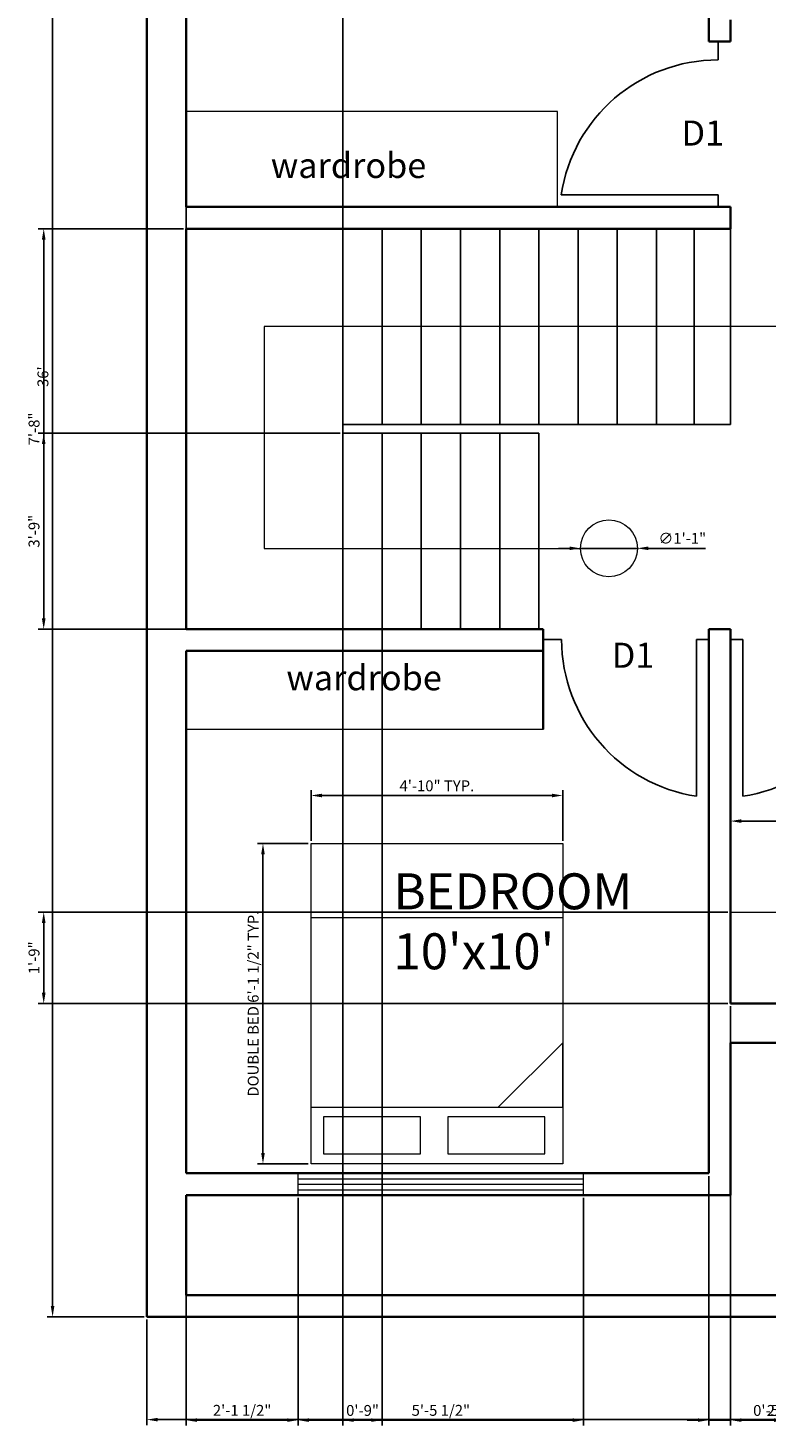
# Model space of a CAD drawing. Units: inches. Extents: x 346 to 762, y 179 to 666.
# Tile 1 of 3: x 348 to 518, y 179 to 500. Entities that reach past the tile are written whole.
import ezdxf

# ---------------------------------------------------------------- set-up
doc = ezdxf.new("R2010")
doc.units = ezdxf.units.IN
for name, color, linetype, lineweight in [('A-ANNO-DIMS', 2, 'Continuous', 18), ('A-ANNO-SYMB', 3, 'Continuous', 18), ('A-ANNO-TEXT', 7, 'Continuous', 18), ('A-AREA-IDEN', 7, 'Continuous', 25), ('A-DOOR', 3, 'Continuous', 25), ('A-FLOR-CASE', 9, 'Continuous', 18), ('A-FLOR-STRS', 7, 'Continuous', 25), ('A-FURN', 8, 'Continuous', 18), ('A-GLAZ', 4, 'Continuous', 18), ('A-WALL', 7, 'Continuous', 35)]:
    doc.layers.add(name, color=color, linetype=linetype, lineweight=lineweight)
doc.styles.get("Standard").update_dxf_attribs({"font": 'arial.ttf'})
doc.dimstyles.new('ISO-25', dxfattribs={"dimtxt": 2.5, "dimasz": 2.5, "dimexe": 1.25, "dimexo": 0.625, "dimtad": 1, "dimdec": 0, "dimlunit": 3, "dimtxsty": 'Standard', "dimcen": 2.5, "dimadec": 0, "dimazin": 0, "dimtfac": 1, "dimtdec": 0, "dimtmove": 0, "dimatfit": 3, "dimfxl": 1, "dimarcsym": 0})

# ---------------------------------------------------------------- blocks, each defined once
blk = doc.blocks.new('*D2')
at = {"layer": 'A-ANNO-DIMS', "color": 0, "lineweight": -2, "transparency": 16777216}
for p, q in [((375.04, 636.22), (352.75, 636.22)), ((354, 633.72), (354, 206.72)), ((375.04, 204.22), (352.75, 204.22))]:
    blk.add_line(p, q, dxfattribs=at)
at = {"layer": 'A-ANNO-DIMS', "color": 0, "transparency": 16777216}
for points in [[(353.58, 633.72), (354.41, 633.72), (354, 636.22)], [(353.58, 206.72), (354.41, 206.72), (354, 204.22)]]:
    blk.add_solid(points, dxfattribs=at)
at = {"layer": 'Defpoints', "color": 0, "transparency": 16777216}
for p in [(375.66, 636.22), (354, 204.22), (375.66, 204.22)]:
    blk.add_point(p, dxfattribs=at)
at = {"layer": 'A-ANNO-DIMS', "color": 0, "transparency": 16777216, "insert": (352.1, 420.22), "char_height": 2.5, "attachment_point": 5, "rotation": 90}
blk.add_mtext("36'", dxfattribs=at)
blk = doc.blocks.new('*D4')
at = {"layer": 'A-ANNO-DIMS', "color": 0, "lineweight": -2, "transparency": 16777216}
for p, q in [((375.66, 203.6), (375.66, 179.38)), ((735.66, 203.6), (735.66, 179.38)), ((378.16, 180.63), (733.16, 180.63))]:
    blk.add_line(p, q, dxfattribs=at)
at = {"layer": 'A-ANNO-DIMS', "color": 0, "transparency": 16777216}
for points in [[(378.16, 181.05), (378.16, 180.21), (375.66, 180.63)], [(733.16, 181.05), (733.16, 180.21), (735.66, 180.63)]]:
    blk.add_solid(points, dxfattribs=at)
at = {"layer": 'Defpoints', "color": 0, "transparency": 16777216}
for p in [(375.66, 204.22), (735.66, 204.22), (735.66, 180.63)]:
    blk.add_point(p, dxfattribs=at)
at = {"layer": 'A-ANNO-DIMS', "color": 0, "transparency": 16777216, "insert": (555.66, 182.53), "char_height": 2.5, "attachment_point": 5}
blk.add_mtext("30'", dxfattribs=at)
blk = doc.blocks.new('BED-DOUBLE')
for p, q in [((0, 0), (0, 73.56)), ((0, 73.56), (57.79, 73.56)), ((57.79, 73.56), (57.79, 0)), ((0, 56.59), (57.79, 56.59)), ((57.79, 27.81), (42.96, 13.04)), ((57.79, 13.04), (57.79, 27.81)), ((0, 0), (0, 13.04)), ((0, 13.04), (57.79, 13.04)), ((57.79, 0), (0, 0))]:
    blk.add_line(p, q)
for points in [[(2.87, 2.28), (25.15, 2.28), (25.15, 10.76), (2.87, 10.76)], [(31.41, 2.28), (53.7, 2.28), (53.7, 10.76), (31.41, 10.76)]]:
    blk.add_lwpolyline(points, close=True)
blk = doc.blocks.new('DOOR-SINGLE-36IN')
for p, q in [((2.79, 36), (0, 36)), ((2.79, 36), (2.79, 0)), ((38, 36), (33.78, 36))]:
    blk.add_line(p, q)
blk.add_arc((-2.63, 36), 36.41, 278.5676, 0)
blk = doc.blocks.new('*D9')
at = {"layer": 'A-ANNO-DIMS', "color": 0, "lineweight": -2, "transparency": 16777216}
for p, q in [((412.71, 312.97), (401.05, 312.97)), ((402.3, 241.91), (402.3, 310.47)), ((412.71, 239.41), (401.05, 239.41))]:
    blk.add_line(p, q, dxfattribs=at)
at = {"layer": 'A-ANNO-DIMS', "color": 0, "transparency": 16777216}
for points in [[(401.88, 310.47), (402.72, 310.47), (402.3, 312.97)], [(401.88, 241.91), (402.72, 241.91), (402.3, 239.41)]]:
    blk.add_solid(points, dxfattribs=at)
at = {"layer": 'Defpoints', "color": 0, "transparency": 16777216}
for p in [(402.3, 312.97), (413.33, 312.97), (413.33, 239.41)]:
    blk.add_point(p, dxfattribs=at)
at = {"layer": 'A-ANNO-DIMS', "color": 0, "transparency": 16777216, "insert": (400.38, 276.19), "char_height": 2.5, "attachment_point": 5, "rotation": 90}
blk.add_mtext('DOUBLE BED 6\'-1 1/2" TYP.', dxfattribs=at)
blk = doc.blocks.new('*D10')
at = {"layer": 'A-ANNO-DIMS', "color": 0, "lineweight": -2, "transparency": 16777216}
for p, q in [((413.33, 313.6), (413.33, 325.26)), ((471.13, 313.6), (471.13, 325.26)), ((415.83, 324.01), (468.63, 324.01))]:
    blk.add_line(p, q, dxfattribs=at)
at = {"layer": 'A-ANNO-DIMS', "color": 0, "transparency": 16777216}
for points in [[(415.83, 324.42), (415.83, 323.59), (413.33, 324.01)], [(468.63, 324.42), (468.63, 323.59), (471.13, 324.01)]]:
    blk.add_solid(points, dxfattribs=at)
at = {"layer": 'Defpoints', "color": 0, "transparency": 16777216}
for p in [(471.13, 324.01), (413.33, 312.97), (471.13, 312.97)]:
    blk.add_point(p, dxfattribs=at)
at = {"layer": 'A-ANNO-DIMS', "color": 0, "transparency": 16777216, "insert": (442.23, 325.91), "char_height": 2.5, "attachment_point": 5}
blk.add_mtext('4\'-10" TYP.', dxfattribs=at)
blk = doc.blocks.new('*D11')
at = {"layer": 'A-ANNO-DIMS', "color": 0, "lineweight": -2, "transparency": 16777216}
for p, q in [((509.66, 323.21), (509.66, 316.88)), ((547.66, 323.21), (547.66, 316.88)), ((512.16, 318.13), (545.16, 318.13)), ((547.66, 318.13), (591.87, 318.13))]:
    blk.add_line(p, q, dxfattribs=at)
at = {"layer": 'A-ANNO-DIMS', "color": 0, "transparency": 16777216}
for points in [[(512.16, 318.55), (512.16, 317.72), (509.66, 318.13)], [(545.16, 318.55), (545.16, 317.72), (547.66, 318.13)]]:
    blk.add_solid(points, dxfattribs=at)
at = {"layer": 'Defpoints', "color": 0, "transparency": 16777216}
for p in [(509.66, 323.83), (547.66, 323.83), (547.66, 318.13)]:
    blk.add_point(p, dxfattribs=at)
at = {"layer": 'A-ANNO-DIMS', "color": 0, "transparency": 16777216, "insert": (571.01, 320.05), "char_height": 2.5, "attachment_point": 5}
blk.add_mtext('SINGLE DOOR 3\'-2" TYP.', dxfattribs=at)
blk = doc.blocks.new('*D17')
at = {"layer": 'A-ANNO-DIMS', "color": 0, "lineweight": -2, "transparency": 16777216}
for p, q in [((509.04, 297.23), (350.71, 297.23)), ((351.96, 278.72), (351.96, 294.73)), ((509.04, 276.22), (350.71, 276.22))]:
    blk.add_line(p, q, dxfattribs=at)
at = {"layer": 'A-ANNO-DIMS', "color": 0, "transparency": 16777216}
for points in [[(351.54, 294.73), (352.38, 294.73), (351.96, 297.23)], [(351.54, 278.72), (352.38, 278.72), (351.96, 276.22)]]:
    blk.add_solid(points, dxfattribs=at)
at = {"layer": 'Defpoints', "color": 0, "transparency": 16777216}
for p in [(351.96, 297.23), (509.66, 297.23), (509.66, 276.22)]:
    blk.add_point(p, dxfattribs=at)
at = {"layer": 'A-ANNO-DIMS', "color": 0, "transparency": 16777216, "insert": (350.06, 286.73), "char_height": 2.5, "attachment_point": 5, "rotation": 90}
blk.add_mtext('1\'-9"', dxfattribs=at)
blk = doc.blocks.new('*D19')
at = {"layer": 'A-ANNO-DIMS', "color": 0, "lineweight": -2, "transparency": 16777216}
for p, q in [((533.83, 279.4), (533.83, 179.27)), ((509.66, 275.6), (509.66, 179.27)), ((512.16, 180.52), (531.33, 180.52))]:
    blk.add_line(p, q, dxfattribs=at)
at = {"layer": 'A-ANNO-DIMS', "color": 0, "transparency": 16777216}
for points in [[(512.16, 180.94), (512.16, 180.11), (509.66, 180.52)], [(531.33, 180.94), (531.33, 180.11), (533.83, 180.52)]]:
    blk.add_solid(points, dxfattribs=at)
at = {"layer": 'Defpoints', "color": 0, "transparency": 16777216}
for p in [(533.83, 280.02), (509.66, 276.22), (533.83, 180.52)]:
    blk.add_point(p, dxfattribs=at)
at = {"layer": 'A-ANNO-DIMS', "color": 0, "transparency": 16777216, "insert": (521.75, 182.42), "char_height": 2.5, "attachment_point": 5}
blk.add_mtext('2\'-0"', dxfattribs=at)
blk = doc.blocks.new('*D24')
at = {"layer": 'A-ANNO-DIMS', "color": 0, "lineweight": -2, "transparency": 16777216}
for p, q in [((509.66, 266.6), (509.66, 179.27)), ((522.15, 266.6), (522.15, 179.27)), ((512.16, 180.52), (519.65, 180.52)), ((522.15, 180.52), (538.14, 180.52))]:
    blk.add_line(p, q, dxfattribs=at)
at = {"layer": 'A-ANNO-DIMS', "color": 0, "transparency": 16777216}
for points in [[(512.16, 180.94), (512.16, 180.11), (509.66, 180.52)], [(519.65, 180.94), (519.65, 180.11), (522.15, 180.52)]]:
    blk.add_solid(points, dxfattribs=at)
at = {"layer": 'Defpoints', "color": 0, "transparency": 16777216}
for p in [(509.66, 267.22), (522.15, 267.22), (522.15, 180.52)]:
    blk.add_point(p, dxfattribs=at)
at = {"layer": 'A-ANNO-DIMS', "color": 0, "transparency": 16777216, "insert": (531.4, 182.44), "char_height": 2.5, "attachment_point": 5}
blk.add_mtext('1\'-0 1/2"', dxfattribs=at)
blk = doc.blocks.new('*D26')
at = {"layer": 'A-ANNO-DIMS', "color": 0, "lineweight": -2, "transparency": 16777216}
for p, q in [((384.04, 454.22), (350.71, 454.22)), ((351.96, 364.72), (351.96, 451.72)), ((384.04, 362.22), (350.71, 362.22))]:
    blk.add_line(p, q, dxfattribs=at)
at = {"layer": 'A-ANNO-DIMS', "color": 0, "transparency": 16777216}
for points in [[(351.54, 451.72), (352.38, 451.72), (351.96, 454.22)], [(351.54, 364.72), (352.38, 364.72), (351.96, 362.22)]]:
    blk.add_solid(points, dxfattribs=at)
at = {"layer": 'Defpoints', "color": 0, "transparency": 16777216}
for p in [(351.96, 454.22), (384.66, 454.22), (384.66, 362.22)]:
    blk.add_point(p, dxfattribs=at)
at = {"layer": 'A-ANNO-DIMS', "color": 0, "transparency": 16777216, "insert": (350.06, 408.22), "char_height": 2.5, "attachment_point": 5, "rotation": 90}
blk.add_mtext('7\'-8"', dxfattribs=at)
blk = doc.blocks.new('*D27')
at = {"layer": 'A-ANNO-DIMS', "color": 0, "lineweight": -2, "transparency": 16777216}
for p, q in [((420.66, 406.6), (420.66, 179.27)), ((429.66, 406.6), (429.66, 179.27)), ((423.16, 180.52), (427.16, 180.52))]:
    blk.add_line(p, q, dxfattribs=at)
at = {"layer": 'A-ANNO-DIMS', "color": 0, "transparency": 16777216}
for points in [[(423.16, 180.94), (423.16, 180.11), (420.66, 180.52)], [(427.16, 180.94), (427.16, 180.11), (429.66, 180.52)]]:
    blk.add_solid(points, dxfattribs=at)
at = {"layer": 'Defpoints', "color": 0, "transparency": 16777216}
for p in [(420.66, 407.22), (429.66, 407.22), (429.66, 180.52)]:
    blk.add_point(p, dxfattribs=at)
at = {"layer": 'A-ANNO-DIMS', "color": 0, "transparency": 16777216, "insert": (425.16, 182.42), "char_height": 2.5, "attachment_point": 5}
blk.add_mtext('0\'-9"', dxfattribs=at)
blk = doc.blocks.new('*D28')
at = {"layer": 'A-ANNO-DIMS', "color": 0, "lineweight": -2, "transparency": 16777216}
for p, q in [((420.04, 407.22), (350.71, 407.22)), ((351.96, 364.72), (351.96, 404.72)), ((420.04, 362.22), (350.71, 362.22))]:
    blk.add_line(p, q, dxfattribs=at)
at = {"layer": 'A-ANNO-DIMS', "color": 0, "transparency": 16777216}
for points in [[(351.54, 404.72), (352.38, 404.72), (351.96, 407.22)], [(351.54, 364.72), (352.38, 364.72), (351.96, 362.22)]]:
    blk.add_solid(points, dxfattribs=at)
at = {"layer": 'Defpoints', "color": 0, "transparency": 16777216}
for p in [(351.96, 407.22), (420.66, 407.22), (420.66, 362.22)]:
    blk.add_point(p, dxfattribs=at)
at = {"layer": 'A-ANNO-DIMS', "color": 0, "transparency": 16777216, "insert": (350.06, 384.72), "char_height": 2.5, "attachment_point": 5, "rotation": 90}
blk.add_mtext('3\'-9"', dxfattribs=at)
blk = doc.blocks.new('*D29')
at = {"layer": 'A-ANNO-DIMS', "color": 0, "lineweight": -2, "transparency": 16777216}
for p, q in [((384.66, 362.85), (384.66, 661.17)), ((387.16, 659.92), (418.16, 659.92)), ((420.66, 362.85), (420.66, 661.17))]:
    blk.add_line(p, q, dxfattribs=at)
at = {"layer": 'A-ANNO-DIMS', "color": 0, "transparency": 16777216}
for points in [[(387.16, 660.34), (387.16, 659.51), (384.66, 659.92)], [(418.16, 660.34), (418.16, 659.51), (420.66, 659.92)]]:
    blk.add_solid(points, dxfattribs=at)
at = {"layer": 'Defpoints', "color": 0, "transparency": 16777216}
for p in [(420.66, 659.92), (384.66, 362.22), (420.66, 362.22)]:
    blk.add_point(p, dxfattribs=at)
at = {"layer": 'A-ANNO-DIMS', "color": 0, "transparency": 16777216, "insert": (402.66, 661.82), "char_height": 2.5, "attachment_point": 5}
blk.add_mtext('3\'-0"', dxfattribs=at)
blk = doc.blocks.new('*D41')
at = {"layer": 'A-ANNO-DIMS', "color": 0, "lineweight": -2, "transparency": 16777216}
for p, q in [((384.66, 231.6), (384.66, 179.27)), ((410.37, 231.6), (410.37, 179.27)), ((387.16, 180.52), (407.87, 180.52))]:
    blk.add_line(p, q, dxfattribs=at)
at = {"layer": 'A-ANNO-DIMS', "color": 0, "transparency": 16777216}
for points in [[(387.16, 180.94), (387.16, 180.11), (384.66, 180.52)], [(407.87, 180.94), (407.87, 180.11), (410.37, 180.52)]]:
    blk.add_solid(points, dxfattribs=at)
at = {"layer": 'Defpoints', "color": 0, "transparency": 16777216}
for p in [(384.66, 232.22), (410.37, 232.22), (410.37, 180.52)]:
    blk.add_point(p, dxfattribs=at)
at = {"layer": 'A-ANNO-DIMS', "color": 0, "transparency": 16777216, "insert": (397.51, 182.44), "char_height": 2.5, "attachment_point": 5}
blk.add_mtext('2\'-1 1/2"', dxfattribs=at)
blk = doc.blocks.new('*D42')
at = {"layer": 'A-ANNO-DIMS', "color": 0, "lineweight": -2, "transparency": 16777216}
for p, q in [((410.37, 231.6), (410.37, 179.27)), ((475.92, 231.6), (475.92, 179.27)), ((412.87, 180.52), (473.42, 180.52))]:
    blk.add_line(p, q, dxfattribs=at)
at = {"layer": 'A-ANNO-DIMS', "color": 0, "transparency": 16777216}
for points in [[(412.87, 180.94), (412.87, 180.11), (410.37, 180.52)], [(473.42, 180.94), (473.42, 180.11), (475.92, 180.52)]]:
    blk.add_solid(points, dxfattribs=at)
at = {"layer": 'Defpoints', "color": 0, "transparency": 16777216}
for p in [(410.37, 232.22), (475.92, 232.22), (475.92, 180.52)]:
    blk.add_point(p, dxfattribs=at)
at = {"layer": 'A-ANNO-DIMS', "color": 0, "transparency": 16777216, "insert": (443.14, 182.44), "char_height": 2.5, "attachment_point": 5}
blk.add_mtext('5\'-5 1/2"', dxfattribs=at)
blk = doc.blocks.new('*D47')
at = {"layer": 'A-ANNO-DIMS', "color": 0, "lineweight": -2, "transparency": 16777216}
for p, q in [((504.66, 236.6), (504.66, 179.27)), ((509.66, 231.6), (509.66, 179.27)), ((502.16, 180.52), (499.66, 180.52)), ((504.66, 180.52), (509.66, 180.52)), ((512.16, 180.52), (522.56, 180.52))]:
    blk.add_line(p, q, dxfattribs=at)
at = {"layer": 'A-ANNO-DIMS', "color": 0, "transparency": 16777216}
for points in [[(502.16, 180.94), (502.16, 180.11), (504.66, 180.52)], [(512.16, 180.94), (512.16, 180.11), (509.66, 180.52)]]:
    blk.add_solid(points, dxfattribs=at)
at = {"layer": 'Defpoints', "color": 0, "transparency": 16777216}
for p in [(504.66, 237.22), (509.66, 232.22), (509.66, 180.52)]:
    blk.add_point(p, dxfattribs=at)
at = {"layer": 'A-ANNO-DIMS', "color": 0, "transparency": 16777216, "insert": (518.61, 182.42), "char_height": 2.5, "attachment_point": 5}
blk.add_mtext('0\'-5"', dxfattribs=at)
blk = doc.blocks.new('*D50')
at = {"layer": 'A-ANNO-DIMS', "color": 0, "lineweight": -2, "transparency": 16777216}
for p, q in [((472.68, 380.79), (470.18, 380.79)), ((475.18, 380.79), (488.27, 380.79)), ((503.89, 380.79), (490.77, 380.79))]:
    blk.add_line(p, q, dxfattribs=at)
at = {"layer": 'A-ANNO-DIMS', "color": 0, "transparency": 16777216}
for points in [[(472.68, 381.21), (472.68, 380.38), (475.18, 380.79)], [(490.77, 381.21), (490.77, 380.38), (488.27, 380.79)]]:
    blk.add_solid(points, dxfattribs=at)
at = {"layer": 'Defpoints', "color": 0, "transparency": 16777216}
for p in [(475.18, 380.79), (488.27, 380.79)]:
    blk.add_point(p, dxfattribs=at)
at = {"layer": 'A-ANNO-DIMS', "color": 0, "transparency": 16777216, "insert": (498.58, 382.76), "char_height": 2.5, "attachment_point": 5, "rotation": 359.9991}
blk.add_mtext('∅1\'-1"', dxfattribs=at)

msp = doc.modelspace()

# ---------------------------------------------------------------- linework, layer by layer
at = {"layer": 'A-ANNO-SYMB'}
for p, q in [((529.92, 431.72), (402.56, 431.72)), ((402.56, 431.72), (402.56, 380.79)), ((402.56, 380.79), (475.18, 380.79))]:
    msp.add_line(p, q, dxfattribs=at)
msp.add_circle((481.73, 380.79), 6.54, dxfattribs=at)
at = {"layer": 'A-FLOR-CASE'}
for p, q in [((469.89, 481.11), (384.66, 481.11)), ((469.89, 459.22), (469.89, 481.11)), ((384.69, 339.22), (466.69, 339.22)), ((509.66, 297.23), (584.3, 297.23))]:
    msp.add_line(p, q, dxfattribs=at)
at = {"layer": 'A-FLOR-STRS'}
for p, q in [((420.66, 409.22), (420.66, 454.22)), ((429.66, 409.22), (429.66, 454.22)), ((438.66, 409.22), (438.66, 454.22)), ((447.66, 409.22), (447.66, 454.22)), ((456.66, 409.22), (456.66, 454.22)), ((465.66, 409.22), (465.66, 454.22)), ((474.66, 409.22), (474.66, 454.22)), ((474.66, 409.22), (474.66, 454.22)), ((483.66, 409.22), (483.66, 454.22)), ((492.66, 409.22), (492.66, 454.22)), ((501.32, 409.22), (501.32, 454.22)), ((509.66, 409.22), (509.66, 454.22)), ((420.66, 362.22), (420.66, 409.22)), ((420.66, 409.22), (509.66, 409.22)), ((420.66, 407.22), (465.66, 407.22)), ((429.66, 362.22), (429.66, 407.22)), ((438.66, 362.22), (438.66, 407.22)), ((447.66, 362.22), (447.66, 407.22)), ((456.66, 362.22), (456.66, 407.22)), ((465.66, 362.22), (465.66, 407.22))]:
    msp.add_line(p, q, dxfattribs=at)
at = {"layer": 'A-GLAZ'}
for p, q in [((410.37, 232.22), (410.37, 237.22)), ((410.37, 235.94), (475.92, 235.94)), ((475.92, 232.22), (475.92, 237.22)), ((410.37, 234.72), (475.92, 234.72)), ((410.37, 233.43), (475.92, 233.43))]:
    msp.add_line(p, q, dxfattribs=at)
at = {"layer": 'A-WALL'}
for p, q in [((375.66, 204.22), (375.66, 636.22)), ((384.66, 459.22), (384.66, 627.22)), ((504.66, 497.22), (504.66, 507.22)), ((509.66, 497.22), (509.66, 502.22)), ((509.66, 497.22), (504.66, 497.22)), ((384.66, 459.22), (509.66, 459.22)), ((509.66, 454.22), (509.66, 459.22)), ((384.66, 454.22), (509.66, 454.22)), ((384.66, 362.22), (384.66, 454.22)), ((384.66, 362.22), (466.66, 362.22)), ((466.66, 339.22), (466.66, 362.22)), ((504.66, 357.22), (504.66, 362.22)), ((504.66, 362.22), (509.66, 362.22)), ((509.66, 276.22), (509.66, 362.22)), ((384.66, 357.22), (466.66, 357.22)), ((384.66, 237.22), (384.66, 357.22)), ((504.66, 237.22), (504.66, 357.22)), ((509.66, 276.22), (601.66, 276.22)), ((509.66, 232.22), (509.66, 267.22)), ((509.66, 267.22), (606.66, 267.22)), ((384.66, 237.22), (504.66, 237.22)), ((384.66, 209.22), (384.66, 232.22)), ((384.66, 232.22), (509.66, 232.22)), ((509.66, 209.22), (384.66, 209.22)), ((509.66, 209.22), (606.66, 209.22)), ((735.66, 204.22), (375.66, 204.22))]:
    msp.add_line(p, q, dxfattribs=at)

# ---------------------------------------------------------------- block references
at = {"layer": 'A-DOOR', "extrusion": (0, 0, -1), "zscale": -1, "rotation": 90.0000000000007}
msp.add_blockref('DOOR-SINGLE-36IN', (-470.79, 459.22), dxfattribs=at)
at = {"layer": 'A-DOOR', "extrusion": (0, 0, -1), "zscale": -1}
msp.add_blockref('DOOR-SINGLE-36IN', (-504.66, 323.83), dxfattribs=at)
at = {"layer": 'A-DOOR'}
msp.add_blockref('DOOR-SINGLE-36IN', (509.66, 323.83), dxfattribs=at)
at = {"layer": 'A-FURN'}
msp.add_blockref('BED-DOUBLE', (413.33, 239.41), dxfattribs=at)

# ---------------------------------------------------------------- texts
at = {"layer": 'A-ANNO-TEXT', "char_height": 5.764, "attachment_point": 1}
for s, insert in [('D1', (498.4, 479.07)), ('wardrobe', (404.1, 471.63)), ('D1', (482.39, 359.11)), ('wardrobe', (407.67, 353.95))]:
    msp.add_mtext_dynamic_manual_height_columns(s, width=202.5556, gutter_width=28.82, heights=[0], dxfattribs=dict(at, insert=insert))
at = {"layer": 'A-AREA-IDEN', "insert": (432.27, 306.13), "char_height": 8.263, "attachment_point": 1}
msp.add_mtext_dynamic_manual_height_columns("BEDROOM\\P10'x10'", width=290.4031, gutter_width=41.32, heights=[0], dxfattribs=at)

# ---------------------------------------------------------------- dimensions: what is measured, and where the dimension line sits
at = {"layer": 'A-ANNO-DIMS'}
for base, p1, p2, override, picture, middle in [((420.66, 659.92), (384.66, 362.22), (420.66, 362.22), {"dimdec": 1, "dimlfac": 1, "dimrnd": 0, "dimzin": 1, "dimdsep": 46, "dimlunit": 4, "dimfrac": 2}, '*D29', (402.66, 661.82)), ((429.66, 180.52), (420.66, 407.22), (429.66, 407.22), {"dimdec": 1, "dimlfac": 1, "dimrnd": 0, "dimzin": 1, "dimdsep": 46, "dimlunit": 4, "dimfrac": 2}, '*D27', (425.16, 182.42)), ((533.83, 180.52), (509.66, 276.22), (533.83, 280.02), {"dimdec": 1, "dimlfac": 1, "dimrnd": 0, "dimzin": 1, "dimdsep": 46, "dimlunit": 4, "dimfrac": 2}, '*D19', (521.75, 182.42)), ((522.15, 180.52), (509.66, 267.22), (522.15, 267.22), {"dimdec": 1, "dimlfac": 1, "dimrnd": 0, "dimzin": 1, "dimdsep": 46, "dimlunit": 4, "dimfrac": 2}, '*D24', (531.4, 182.44)), ((509.66, 180.52), (504.66, 237.22), (509.66, 232.22), {"dimdec": 1, "dimlfac": 1, "dimrnd": 0, "dimzin": 1, "dimdsep": 46, "dimlunit": 4, "dimfrac": 2}, '*D47', (518.61, 182.42)), ((410.37, 180.52), (384.66, 232.22), (410.37, 232.22), {"dimdec": 1, "dimlfac": 1, "dimrnd": 0, "dimzin": 1, "dimdsep": 46, "dimlunit": 4, "dimfrac": 2}, '*D41', (397.51, 182.44)), ((475.917, 180.5219), (410.3665, 232.2219), (475.917, 232.2219), {"dimdec": 1, "dimlfac": 1, "dimrnd": 0, "dimzin": 1, "dimdsep": 46, "dimlunit": 4, "dimfrac": 2}, '*D42', (443.1418, 182.4395)), ((735.66, 180.63), (375.66, 204.22), (735.66, 204.22), {"dimclrd": 0, "dimclre": 0, "dimclrt": 0}, '*D4', (555.66, 182.53))]:
    dim = msp.add_linear_dim(base=base, p1=p1, p2=p2, dimstyle='ISO-25', override=override, dxfattribs=at)
    dim.commit()
    dim.dimension.update_dxf_attribs({"geometry": picture, "text_midpoint": middle})
for base, p1, p2, override, picture, middle in [((354, 204.22), (375.66, 636.22), (375.66, 204.22), {"dimclrd": 0, "dimclre": 0, "dimclrt": 0}, '*D2', (352.1, 420.22)), ((351.96, 454.22), (384.66, 362.22), (384.66, 454.22), {"dimdec": 1, "dimlfac": 1, "dimrnd": 0, "dimzin": 1, "dimdsep": 46, "dimlunit": 4, "dimfrac": 2}, '*D26', (350.06, 408.22)), ((351.96, 407.22), (420.66, 362.22), (420.66, 407.22), {"dimdec": 1, "dimlfac": 1, "dimrnd": 0, "dimzin": 1, "dimdsep": 46, "dimlunit": 4, "dimfrac": 2}, '*D28', (350.06, 384.72)), ((351.96, 297.23), (509.66, 276.22), (509.66, 297.23), {"dimdec": 1, "dimlfac": 1, "dimrnd": 0, "dimzin": 1, "dimdsep": 46, "dimlunit": 4, "dimfrac": 2}, '*D17', (350.06, 286.73))]:
    dim = msp.add_linear_dim(base=base, p1=p1, p2=p2, angle=90, dimstyle='ISO-25', override=override, dxfattribs=at)
    dim.commit()
    dim.dimension.update_dxf_attribs({"geometry": picture, "text_midpoint": middle})
dim = msp.add_diameter_dim_2p(p1=(475.18, 380.79), p2=(488.27, 380.79), dimstyle='ISO-25', override={"dimdec": 1, "dimlfac": 1, "dimrnd": 0, "dimzin": 1, "dimdsep": 46, "dimlunit": 4, "dimfrac": 2}, dxfattribs=at)
dim.commit()
dim.dimension.update_dxf_attribs({"geometry": '*D50', "text_midpoint": (498.58, 380.79), "dimtype": 163})
for base, p1, p2, text, picture, middle in [((471.13, 324.01), (413.33, 312.97), (471.13, 312.97), '<> TYP.', '*D10', (442.23, 325.91)), ((547.66, 318.13), (509.66, 323.83), (547.66, 323.83), 'SINGLE DOOR <> TYP.', '*D11', (571.01, 320.05))]:
    dim = msp.add_linear_dim(base=base, p1=p1, p2=p2, text=text, dimstyle='ISO-25', override={"dimdec": 1, "dimlfac": 1, "dimrnd": 0, "dimzin": 1, "dimdsep": 46, "dimlunit": 4, "dimfrac": 2}, dxfattribs=at)
    dim.commit()
    dim.dimension.update_dxf_attribs({"geometry": picture, "text_midpoint": middle})
dim = msp.add_linear_dim(base=(402.3, 312.97), p1=(413.33, 239.41), p2=(413.33, 312.97), angle=90, text='DOUBLE BED <> TYP.', dimstyle='ISO-25', override={"dimdec": 1, "dimlfac": 1, "dimrnd": 0, "dimzin": 1, "dimdsep": 46, "dimlunit": 4, "dimfrac": 2}, dxfattribs=at)
dim.commit()
dim.dimension.update_dxf_attribs({"geometry": '*D9', "text_midpoint": (400.38, 276.19)})

doc.saveas('drawing.dxf')
